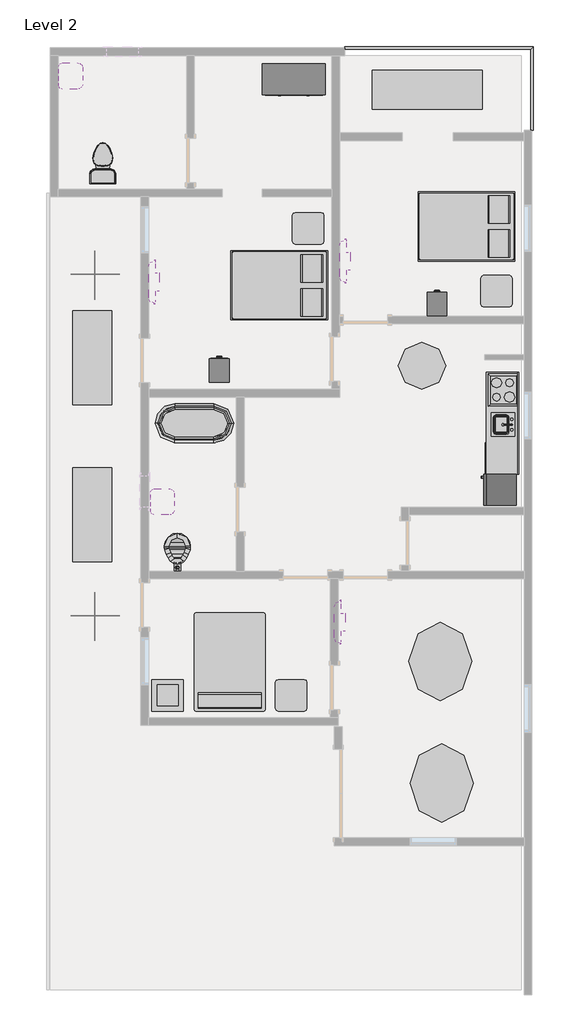
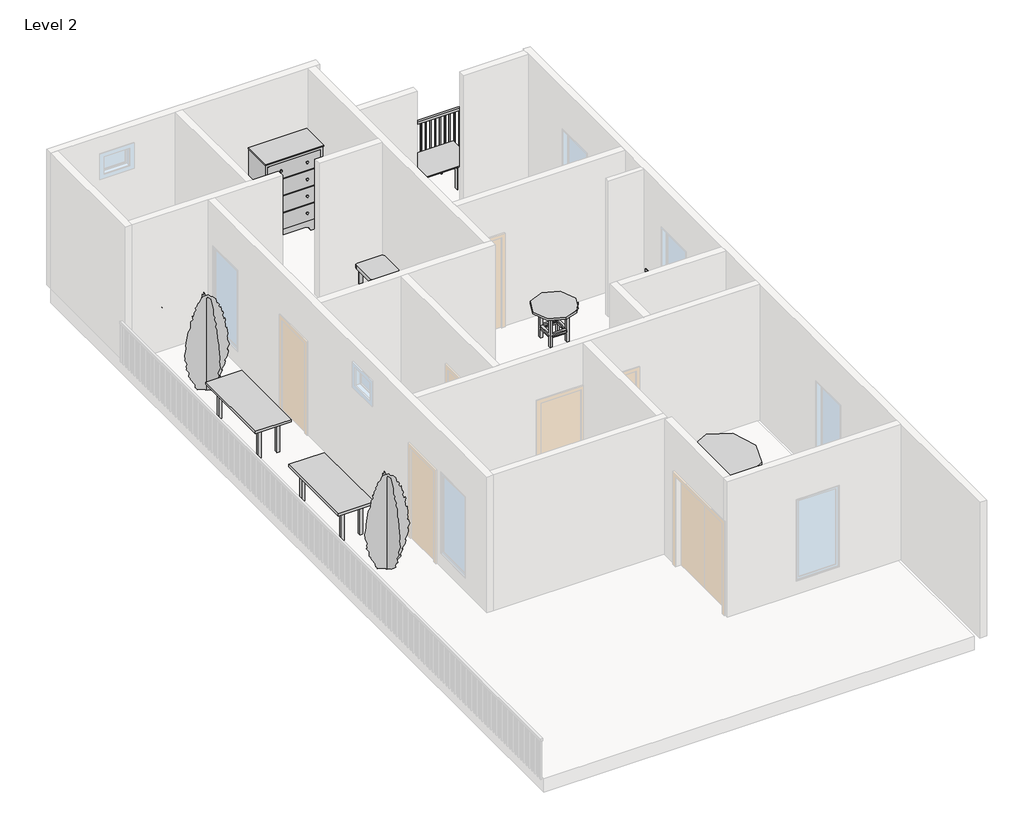
# One storey, part 4 of 4: 20 furniture elements, 6 flow terminals, 4 proxies, 2 geographic elements, 1 railing.
"""IFC4 building model written with IfcOpenShell, lengths in millimetres."""

from ifc_helpers import new_model, si_unit, frame, origin, place, context, project, spatial, polyline, outline, extrude, faceted_brep, transform, mapped, element, save
from components import proxy_a6faaae8, proxy_45b28599, kitchenette_medium_kitchenette_medium_844211aa, proxy_c523a7b7, flow_terminal_871c2e40, flow_terminal_62a433f7, flow_terminal_6d55091a, toilet_domestic_3d_toilet_domestic_3d_f7549cf7, toilet_domestic_3d_toilet_domestic_3d_183bbd19, flow_terminal_b374fae2, furniture_0810mm_56245f3a, furniture_c8abb964, furniture_0253826f, furniture_b1353b55, furniture_c6510c7c, furniture_9fa109b2, furniture_b5c51a22, furniture_92191dda, furniture_905aceb5, furniture_743965d2, furniture_bcf351fa, furniture_a5b052b6, rpc_tree_conifer_0001_chinese_juniper_7_1b9786cd

model = new_model("IFC4")

# Units and contexts
model_context = context("Model", 3, world=origin())
ifc_project = project(units=[si_unit("LENGTHUNIT", "METRE", prefix="MILLI")], contexts=[model_context])

# Site, building, storey
site = spatial("IfcSite", under=ifc_project)
building = spatial("IfcBuilding", under=site)
storey = spatial("IfcBuildingStorey", under=building, Name="Level 2", Elevation=3048.0)

# Proxies
placement = place(None, origin())
proxy_shape = proxy_a6faaae8(model_context)
element("IfcBuildingElementProxy", 1, Name="Cook Top-4 Unit2 : 22\" x 20\"", ObjectType="Cook Top-4 Unit2 : 22\" x 20\"", at=placement, inside=storey, context=model_context, shape_type="MappedRepresentation", body=[
    mapped(proxy_shape, transform((-3246.660887, 7038.0910469, 3048.0), x_axis=(0.0, -1.0, 0.0), y_axis=(1.0, 0.0, 0.0), z_axis=(0.0, 0.0, 1.0))),
])
proxy_2_shape = proxy_45b28599(model_context)
element("IfcBuildingElementProxy", 2, Name="Dishwasher : 24\" x 24\" x 34\"", ObjectType="Dishwasher : 24\" x 24\" x 34\"", at=placement, inside=storey, context=model_context, shape_type="MappedRepresentation", body=[
    mapped(proxy_2_shape, transform((-3538.5104518, 6086.9085154, 3048.0), x_axis=(0.0, -1.0, 0.0), y_axis=(1.0, 0.0, 0.0), z_axis=(0.0, 0.0, 1.0))),
])
kitchenette_medium_kitchenette_medium_shape = kitchenette_medium_kitchenette_medium_844211aa(model_context)
element("IfcBuildingElementProxy", 3, Name="Kitchenette - Medium : Kitchenette - Medium", ObjectType="Kitchenette - Medium : Kitchenette - Medium", at=placement, inside=storey, context=model_context, shape_type="MappedRepresentation", body=[
    mapped(kitchenette_medium_kitchenette_medium_shape, transform((-2941.860887, 6713.9287518, 3048.0), x_axis=(0.0, -1.0, 0.0), y_axis=(1.0, 0.0, 0.0), z_axis=(0.0, 0.0, 1.0))),
])
proxy_3_shape = proxy_c523a7b7(model_context)
element("IfcBuildingElementProxy", 4, Name="Refrigerator : 24\" x 25\" LH", ObjectType="Refrigerator : 24\" x 25\" LH", at=placement, inside=storey, context=model_context, shape_type="MappedRepresentation", body=[
    mapped(proxy_3_shape, transform((-3292.3098585, 5101.3410469, 3048.0), x_axis=(0.0, -1.0, 0.0), y_axis=(1.0, 0.0, 0.0), z_axis=(0.0, 0.0, 1.0))),
])

# Flow terminals
flow_terminal_shape = flow_terminal_871c2e40(model_context)
element("IfcFlowTerminal", 5, ObjectType="Sink Kitchen-Island : 18\" x 18\"", at=placement, inside=storey, context=model_context, shape_type="MappedRepresentation", body=[
    mapped(flow_terminal_shape, transform((-3249.0062881, 6380.6802875, 3033.6), x_axis=(0.0, -1.0, 0.0), y_axis=(1.0, 0.0, 0.0), z_axis=(0.0, 0.0, 1.0))),
])
flow_terminal_2_shape = flow_terminal_62a433f7(model_context)
element("IfcFlowTerminal", 6, ObjectType="Sink Vanity-Square : 20\" x 18\"", at=placement, inside=storey, context=model_context, shape_type="MappedRepresentation", body=[
    mapped(flow_terminal_2_shape, transform((-11689.8154859, 13118.4018063, 3962.4), x_axis=(0.0, 1.0000000000000002, 0.0), y_axis=(-1.0000000000000002, 0.0, 0.0), z_axis=(0.0, 0.0, 1.0))),
])
element("IfcFlowTerminal", 7, ObjectType="Sink Vanity-Square : 20\" x 18\"", at=placement, inside=storey, context=model_context, shape_type="MappedRepresentation", body=[
    mapped(flow_terminal_2_shape, transform((-9911.8154859, 4850.7018063, 3962.4), x_axis=(0.0, 1.0000000000000002, 0.0), y_axis=(-1.0000000000000002, 0.0, 0.0), z_axis=(0.0, 0.0, 1.0))),
])
flow_terminal_3_shape = flow_terminal_6d55091a(model_context)
element("IfcFlowTerminal", 8, ObjectType="Toilet-Commercial-Wall-3D : 15\" Seat Height", at=placement, inside=storey, context=model_context, shape_type="MappedRepresentation", body=[
    mapped(flow_terminal_3_shape, transform((-9976.1640408, 3443.9910469, 3048.0), x_axis=(1.0, 0.0, 0.0), y_axis=(0.0, 1.0, 0.0), z_axis=(0.0, 0.0, 1.0))),
])
toilet_domestic_3d_toilet_domestic_3d_shape = toilet_domestic_3d_toilet_domestic_3d_f7549cf7(model_context)
toilet_domestic_3d_toilet_domestic_3d_2_shape = toilet_domestic_3d_toilet_domestic_3d_183bbd19(model_context)
element("IfcFlowTerminal", 9, ObjectType="Toilet-Domestic-3D : Toilet-Domestic-3D", at=placement, inside=storey, context=model_context, shape_type="MappedRepresentation", body=[
    mapped(toilet_domestic_3d_toilet_domestic_3d_shape, transform((-11019.060887, 11533.2870743, 3048.0), x_axis=(-1.0000000000000004, 0.0, 0.0), y_axis=(0.0, -1.0000000000000004, 0.0), z_axis=(0.0, 0.0, 1.0))),
    mapped(toilet_domestic_3d_toilet_domestic_3d_2_shape, transform((-11019.060887, 11533.2870743, 3048.0), x_axis=(-1.0000000000000004, 0.0, 0.0), y_axis=(0.0, -1.0000000000000004, 0.0), z_axis=(0.0, 0.0, 1.0))),
])
flow_terminal_4_shape = flow_terminal_b374fae2(model_context)
element("IfcFlowTerminal", 10, ObjectType="Tub-Free Standing-3D : 30\" x 60\"", at=placement, inside=storey, context=model_context, shape_type="MappedRepresentation", body=[
    mapped(flow_terminal_4_shape, transform((-9241.060887, 6390.3910469, 3048.0), x_axis=(0.0, 1.0, 0.0), y_axis=(-1.0, 0.0, 0.0), z_axis=(0.0, 0.0, 1.0))),
])

# Furniture
furniture_0810mm_shape = furniture_0810mm_56245f3a(model_context)
element("IfcFurniture", 11, ObjectType="0810mm", at=placement, inside=storey, context=model_context, shape_type="MappedRepresentation", body=[
    mapped(furniture_0810mm_shape, transform((-6464.7222634, 2533.535561, 4267.2), x_axis=(0.0, 0.9999999999999998, 0.0), y_axis=(-0.9999999999999998, 0.0, 0.0), z_axis=(0.0, 0.0, 1.0))),
])
element("IfcFurniture", 12, ObjectType="0810mm", at=placement, inside=storey, context=model_context, shape_type="MappedRepresentation", body=[
    mapped(furniture_0810mm_shape, transform((-10071.5222634, 9137.535561, 4267.2), x_axis=(0.0, 0.9999999999999998, 0.0), y_axis=(-0.9999999999999998, 0.0, 0.0), z_axis=(0.0, 0.0, 1.0))),
])
element("IfcFurniture", 13, ObjectType="0810mm", at=placement, inside=storey, context=model_context, shape_type="MappedRepresentation", body=[
    mapped(furniture_0810mm_shape, transform((-6363.1222634, 9543.935561, 4267.2), x_axis=(0.0, 0.9999999999999998, 0.0), y_axis=(-0.9999999999999998, 0.0, 0.0), z_axis=(0.0, 0.0, 1.0))),
])
furniture_shape = furniture_c8abb964(model_context)
element("IfcFurniture", 14, ObjectType="Bed-Box : Double 53\" x 74\"", at=placement, inside=storey, context=model_context, shape_type="MappedRepresentation", body=[
    mapped(furniture_shape, transform((-7355.6313788, 9409.2435059, 3048.0), x_axis=(0.0, -1.0, 0.0), y_axis=(1.0, 0.0, 0.0), z_axis=(0.0, 0.0, 1.0))),
])
element("IfcFurniture", 15, ObjectType="Bed-Box : Double 53\" x 74\"", at=placement, inside=storey, context=model_context, shape_type="MappedRepresentation", body=[
    mapped(furniture_shape, transform((-3723.4313788, 10552.2435059, 3048.0), x_axis=(0.0, -1.0, 0.0), y_axis=(1.0, 0.0, 0.0), z_axis=(0.0, 0.0, 1.0))),
])
furniture_2_shape = furniture_0253826f(model_context)
element("IfcFurniture", 16, ObjectType="Bed-Standard : Double 54\" x 75\"", at=placement, inside=storey, context=model_context, shape_type="MappedRepresentation", body=[
    mapped(furniture_2_shape, transform((-8283.7723624, 1709.2959649, 3048.0), x_axis=(-1.0, 0.0, 0.0), y_axis=(0.0, -1.0, 0.0), z_axis=(0.0, 0.0, 1.0))),
])
furniture_3_shape = furniture_b1353b55(model_context)
element("IfcFurniture", 17, ObjectType="Cabinet-File 4 Drawer : 15\" x 18\"", at=placement, inside=storey, context=model_context, shape_type="MappedRepresentation", body=[
    mapped(furniture_3_shape, transform((-8886.3573341, 7276.9567468, 3048.0), x_axis=(-1.0000000000000007, 0.0, 0.0), y_axis=(0.0, -1.0000000000000007, 0.0), z_axis=(0.0, 0.0, 1.0))),
])
element("IfcFurniture", 18, ObjectType="Cabinet-File 4 Drawer : 15\" x 18\"", at=placement, inside=storey, context=model_context, shape_type="MappedRepresentation", body=[
    mapped(furniture_3_shape, transform((-4657.2573341, 8559.6567468, 3048.0), x_axis=(-1.0000000000000004, 0.0, 0.0), y_axis=(0.0, -1.0000000000000004, 0.0), z_axis=(0.0, 0.0, 1.0))),
])
furniture_4_shape = furniture_c6510c7c(model_context)
element("IfcFurniture", 19, ObjectType="Counter Top w Sink Hole : 24\" Depth", at=placement, inside=storey, context=model_context, shape_type="MappedRepresentation", body=[
    mapped(furniture_4_shape, transform((-2941.860887, 6180.5287518, 3033.6), x_axis=(0.0, -1.0, 0.0), y_axis=(1.0, 0.0, 0.0), z_axis=(0.0, 0.0, 1.0))),
])
furniture_5_shape = furniture_9fa109b2(model_context)
element("IfcFurniture", 20, ObjectType="Dresser : 48\" x 72\" x 24\"", at=placement, inside=storey, context=model_context, shape_type="MappedRepresentation", body=[
    mapped(furniture_5_shape, transform((-7041.4676272, 13433.754001, 3048.0), x_axis=(1.0, 0.0, 0.0), y_axis=(0.0, 1.0, 0.0), z_axis=(0.0, 0.0, 1.0))),
])
furniture_6_shape = furniture_b5c51a22(model_context)
element("IfcFurniture", 21, ObjectType="Table-Coffee : 24\" x 24\" x 24\"", at=placement, inside=storey, context=model_context, shape_type="MappedRepresentation", body=[
    mapped(furniture_6_shape, transform((-9780.0266537, 1011.9799691, 3048.0), x_axis=(1.0, 0.0, 0.0), y_axis=(0.0, 1.0, 0.0), z_axis=(0.0, 0.0, 1.0))),
])
furniture_7_shape = furniture_92191dda(model_context)
element("IfcFurniture", 22, ObjectType="Table-Dining : 30\" x 84\" x 22\"", at=placement, inside=storey, context=model_context, shape_type="MappedRepresentation", body=[
    mapped(furniture_7_shape, transform((-4738.1266537, 12772.1799691, 3048.0), x_axis=(1.0, 0.0, 0.0), y_axis=(0.0, 1.0, 0.0), z_axis=(0.0, 0.0, 1.0))),
])
furniture_8_shape = furniture_905aceb5(model_context)
element("IfcFurniture", 23, ObjectType="Table-Dining Round w Chairs : 36\" Diameter", at=placement, inside=storey, context=model_context, shape_type="MappedRepresentation", body=[
    mapped(furniture_8_shape, transform((-4925.1428542, 7692.8697354, 3048.0), x_axis=(1.0, 0.0, 0.0), y_axis=(0.0, 1.0, 0.0), z_axis=(0.0, 0.0, 1.0))),
])
furniture_9_shape = furniture_743965d2(model_context)
element("IfcFurniture", 24, ObjectType="Table-Ellipse : 60\" x 48\"", at=placement, inside=storey, context=model_context, shape_type="MappedRepresentation", body=[
    mapped(furniture_9_shape, transform((-4465.860887, 1767.5910469, 3048.0), x_axis=(0.0, 1.0000000000000002, 0.0), y_axis=(-1.0000000000000002, 0.0, 0.0), z_axis=(0.0, 0.0, 1.0))),
])
element("IfcFurniture", 25, ObjectType="Table-Ellipse : 60\" x 48\"", at=placement, inside=storey, context=model_context, shape_type="MappedRepresentation", body=[
    mapped(furniture_9_shape, transform((-4440.460887, -594.6089531, 3048.0), x_axis=(0.0, 1.0000000000000002, 0.0), y_axis=(-1.0000000000000002, 0.0, 0.0), z_axis=(0.0, 0.0, 1.0))),
])
furniture_10_shape = furniture_bcf351fa(model_context)
element("IfcFurniture", 26, ObjectType="Table-End : 24\" x 24\"", at=placement, inside=storey, context=model_context, shape_type="MappedRepresentation", body=[
    mapped(furniture_10_shape, transform((-3682.1945173, 8803.3910469, 3048.0), x_axis=(1.0, 0.0, 0.0), y_axis=(0.0, 1.0, 0.0), z_axis=(0.0, 0.0, 1.0))),
])
element("IfcFurniture", 27, ObjectType="Table-End : 24\" x 24\"", at=placement, inside=storey, context=model_context, shape_type="MappedRepresentation", body=[
    mapped(furniture_10_shape, transform((-7339.7945173, 10022.5910469, 3048.0), x_axis=(1.0, 0.0, 0.0), y_axis=(0.0, 1.0, 0.0), z_axis=(0.0, 0.0, 1.0))),
])
element("IfcFurniture", 28, ObjectType="Table-End : 24\" x 24\"", at=placement, inside=storey, context=model_context, shape_type="MappedRepresentation", body=[
    mapped(furniture_10_shape, transform((-7669.9945173, 954.7910469, 3048.0), x_axis=(1.0, 0.0, 0.0), y_axis=(0.0, 1.0, 0.0), z_axis=(0.0, 0.0, 1.0))),
])
furniture_11_shape = furniture_a5b052b6(model_context)
element("IfcFurniture", 29, ObjectType="Table-Rectangular : 72\" x 30\"", at=placement, inside=storey, context=model_context, shape_type="MappedRepresentation", body=[
    mapped(furniture_11_shape, transform((-11222.260887, 7660.3910469, 3048.0), x_axis=(0.0, 1.0, 0.0), y_axis=(-1.0, 0.0, 0.0), z_axis=(0.0, 0.0, 1.0))),
])
element("IfcFurniture", 30, ObjectType="Table-Rectangular : 72\" x 30\"", at=placement, inside=storey, context=model_context, shape_type="MappedRepresentation", body=[
    mapped(furniture_11_shape, transform((-11222.260887, 4612.3910469, 3048.0), x_axis=(0.0, 1.0000000000000002, 0.0), y_axis=(-1.0000000000000002, 0.0, 0.0), z_axis=(0.0, 0.0, 1.0))),
])

# Geographic elements
rpc_tree_conifer_0001_chinese_juniper_7_shape = rpc_tree_conifer_0001_chinese_juniper_7_1b9786cd(model_context)
element("IfcGeographicElement", 31, ObjectType="RPC Tree - Conifer.0001 : Chinese Juniper - 7'", at=placement, inside=storey, context=model_context, shape_type="MappedRepresentation", body=[
    mapped(rpc_tree_conifer_0001_chinese_juniper_7_shape, transform((-11171.6575581, 9285.9910469, 3048.0), x_axis=(1.0, 0.0, 0.0), y_axis=(0.0, 1.0, 0.0), z_axis=(0.0, 0.0, 1.0))),
])
element("IfcGeographicElement", 32, ObjectType="RPC Tree - Conifer.0001 : Chinese Juniper - 7'", at=placement, inside=storey, context=model_context, shape_type="MappedRepresentation", body=[
    mapped(rpc_tree_conifer_0001_chinese_juniper_7_shape, transform((-11171.6575581, 2656.5910469, 3048.0), x_axis=(1.0, 0.0, 0.0), y_axis=(0.0, 1.0, 0.0), z_axis=(0.0, 0.0, 1.0))),
])

# Railing
element("IfcRailing", 33, ObjectType="Handrail - Rectangular", at=placement, inside=storey, context=model_context, shape_type="SolidModel", body=[
    faceted_brep([(-6320.060887, 13705.5910469, 3962.4), (-6320.060887, 13705.5910469, 3911.6), (-6320.060887, 13654.7910469, 3911.6), (-6320.060887, 13654.7910469, 3962.4), (-2662.460887, 13705.5910469, 3962.4), (-2662.460887, 13705.5910469, 3911.6), (-2713.260887, 13654.7910469, 3911.6), (-2713.260887, 13654.7910469, 3962.4), (-2662.460887, 12079.9910469, 3962.4), (-2713.260887, 12079.9910469, 3962.4), (-2713.260887, 12079.9910469, 3911.6), (-2662.460887, 12079.9910469, 3911.6)], [[[0, 1, 2, 3]], [[1, 0, 4, 5]], [[2, 1, 5, 6]], [[3, 2, 6, 7]], [[0, 3, 7, 4]], [[8, 9, 10, 11]], [[5, 4, 8, 11]], [[6, 5, 11, 10]], [[7, 6, 10, 9]], [[4, 7, 9, 8]]]),
    extrude(outline(polyline([(-2697.385887, 12165.7160469), (-2678.335887, 12165.7160469), (-2678.335887, 12146.6660469), (-2697.385887, 12146.6660469), (-2697.385887, 12165.7160469)])), frame((0.0, 0.0, 3048.0), z_axis=(0.0, 0.0, 1.0), x_axis=(1.0, 0.0, 0.0)), (0.0, 0.0, 1.0), 863.6),
    extrude(outline(polyline([(-2697.385887, 12267.3160469), (-2678.335887, 12267.3160469), (-2678.335887, 12248.2660469), (-2697.385887, 12248.2660469), (-2697.385887, 12267.3160469)])), frame((0.0, 0.0, 3048.0), z_axis=(0.0, 0.0, 1.0), x_axis=(1.0, 0.0, 0.0)), (0.0, 0.0, 1.0), 863.6),
    extrude(outline(polyline([(-2697.385887, 12368.9160469), (-2678.335887, 12368.9160469), (-2678.335887, 12349.8660469), (-2697.385887, 12349.8660469), (-2697.385887, 12368.9160469)])), frame((0.0, 0.0, 3048.0), z_axis=(0.0, 0.0, 1.0), x_axis=(1.0, 0.0, 0.0)), (0.0, 0.0, 1.0), 863.6),
    extrude(outline(polyline([(-2697.385887, 12470.5160469), (-2678.335887, 12470.5160469), (-2678.335887, 12451.4660469), (-2697.385887, 12451.4660469), (-2697.385887, 12470.5160469)])), frame((0.0, 0.0, 3048.0), z_axis=(0.0, 0.0, 1.0), x_axis=(1.0, 0.0, 0.0)), (0.0, 0.0, 1.0), 863.6),
    extrude(outline(polyline([(-2697.385887, 12572.1160469), (-2678.335887, 12572.1160469), (-2678.335887, 12553.0660469), (-2697.385887, 12553.0660469), (-2697.385887, 12572.1160469)])), frame((0.0, 0.0, 3048.0), z_axis=(0.0, 0.0, 1.0), x_axis=(1.0, 0.0, 0.0)), (0.0, 0.0, 1.0), 863.6),
    extrude(outline(polyline([(-2697.385887, 12673.7160469), (-2678.335887, 12673.7160469), (-2678.335887, 12654.6660469), (-2697.385887, 12654.6660469), (-2697.385887, 12673.7160469)])), frame((0.0, 0.0, 3048.0), z_axis=(0.0, 0.0, 1.0), x_axis=(1.0, 0.0, 0.0)), (0.0, 0.0, 1.0), 863.6),
    extrude(outline(polyline([(-2697.385887, 12775.3160469), (-2678.335887, 12775.3160469), (-2678.335887, 12756.2660469), (-2697.385887, 12756.2660469), (-2697.385887, 12775.3160469)])), frame((0.0, 0.0, 3048.0), z_axis=(0.0, 0.0, 1.0), x_axis=(1.0, 0.0, 0.0)), (0.0, 0.0, 1.0), 863.6),
    extrude(outline(polyline([(-2697.385887, 12876.9160469), (-2678.335887, 12876.9160469), (-2678.335887, 12857.8660469), (-2697.385887, 12857.8660469), (-2697.385887, 12876.9160469)])), frame((0.0, 0.0, 3048.0), z_axis=(0.0, 0.0, 1.0), x_axis=(1.0, 0.0, 0.0)), (0.0, 0.0, 1.0), 863.6),
    extrude(outline(polyline([(-2697.385887, 12978.5160469), (-2678.335887, 12978.5160469), (-2678.335887, 12959.4660469), (-2697.385887, 12959.4660469), (-2697.385887, 12978.5160469)])), frame((0.0, 0.0, 3048.0), z_axis=(0.0, 0.0, 1.0), x_axis=(1.0, 0.0, 0.0)), (0.0, 0.0, 1.0), 863.6),
    extrude(outline(polyline([(-2697.385887, 13080.1160469), (-2678.335887, 13080.1160469), (-2678.335887, 13061.0660469), (-2697.385887, 13061.0660469), (-2697.385887, 13080.1160469)])), frame((0.0, 0.0, 3048.0), z_axis=(0.0, 0.0, 1.0), x_axis=(1.0, 0.0, 0.0)), (0.0, 0.0, 1.0), 863.6),
    extrude(outline(polyline([(-2697.385887, 13181.7160469), (-2678.335887, 13181.7160469), (-2678.335887, 13162.6660469), (-2697.385887, 13162.6660469), (-2697.385887, 13181.7160469)])), frame((0.0, 0.0, 3048.0), z_axis=(0.0, 0.0, 1.0), x_axis=(1.0, 0.0, 0.0)), (0.0, 0.0, 1.0), 863.6),
    extrude(outline(polyline([(-2697.385887, 13283.3160469), (-2678.335887, 13283.3160469), (-2678.335887, 13264.2660469), (-2697.385887, 13264.2660469), (-2697.385887, 13283.3160469)])), frame((0.0, 0.0, 3048.0), z_axis=(0.0, 0.0, 1.0), x_axis=(1.0, 0.0, 0.0)), (0.0, 0.0, 1.0), 863.6),
    extrude(outline(polyline([(-2697.385887, 13384.9160469), (-2678.335887, 13384.9160469), (-2678.335887, 13365.8660469), (-2697.385887, 13365.8660469), (-2697.385887, 13384.9160469)])), frame((0.0, 0.0, 3048.0), z_axis=(0.0, 0.0, 1.0), x_axis=(1.0, 0.0, 0.0)), (0.0, 0.0, 1.0), 863.6),
    extrude(outline(polyline([(-2697.385887, 13486.5160469), (-2678.335887, 13486.5160469), (-2678.335887, 13467.4660469), (-2697.385887, 13467.4660469), (-2697.385887, 13486.5160469)])), frame((0.0, 0.0, 3048.0), z_axis=(0.0, 0.0, 1.0), x_axis=(1.0, 0.0, 0.0)), (0.0, 0.0, 1.0), 863.6),
    extrude(outline(polyline([(-2697.385887, 13588.1160469), (-2678.335887, 13588.1160469), (-2678.335887, 13569.0660469), (-2697.385887, 13569.0660469), (-2697.385887, 13588.1160469)])), frame((0.0, 0.0, 3048.0), z_axis=(0.0, 0.0, 1.0), x_axis=(1.0, 0.0, 0.0)), (0.0, 0.0, 1.0), 863.6),
    extrude(outline(polyline([(-2773.585887, 13670.6660469), (-2773.585887, 13689.7160469), (-2754.535887, 13689.7160469), (-2754.535887, 13670.6660469), (-2773.585887, 13670.6660469)])), frame((0.0, 0.0, 3048.0), z_axis=(0.0, 0.0, 1.0), x_axis=(1.0, 0.0, 0.0)), (0.0, 0.0, 1.0), 863.6),
    extrude(outline(polyline([(-2875.185887, 13670.6660469), (-2875.185887, 13689.7160469), (-2856.135887, 13689.7160469), (-2856.135887, 13670.6660469), (-2875.185887, 13670.6660469)])), frame((0.0, 0.0, 3048.0), z_axis=(0.0, 0.0, 1.0), x_axis=(1.0, 0.0, 0.0)), (0.0, 0.0, 1.0), 863.6),
    extrude(outline(polyline([(-2976.785887, 13670.6660469), (-2976.785887, 13689.7160469), (-2957.735887, 13689.7160469), (-2957.735887, 13670.6660469), (-2976.785887, 13670.6660469)])), frame((0.0, 0.0, 3048.0), z_axis=(0.0, 0.0, 1.0), x_axis=(1.0, 0.0, 0.0)), (0.0, 0.0, 1.0), 863.6),
    extrude(outline(polyline([(-3078.385887, 13670.6660469), (-3078.385887, 13689.7160469), (-3059.335887, 13689.7160469), (-3059.335887, 13670.6660469), (-3078.385887, 13670.6660469)])), frame((0.0, 0.0, 3048.0), z_axis=(0.0, 0.0, 1.0), x_axis=(1.0, 0.0, 0.0)), (0.0, 0.0, 1.0), 863.6),
    extrude(outline(polyline([(-3179.985887, 13670.6660469), (-3179.985887, 13689.7160469), (-3160.935887, 13689.7160469), (-3160.935887, 13670.6660469), (-3179.985887, 13670.6660469)])), frame((0.0, 0.0, 3048.0), z_axis=(0.0, 0.0, 1.0), x_axis=(1.0, 0.0, 0.0)), (0.0, 0.0, 1.0), 863.6),
    extrude(outline(polyline([(-3281.585887, 13670.6660469), (-3281.585887, 13689.7160469), (-3262.535887, 13689.7160469), (-3262.535887, 13670.6660469), (-3281.585887, 13670.6660469)])), frame((0.0, 0.0, 3048.0), z_axis=(0.0, 0.0, 1.0), x_axis=(1.0, 0.0, 0.0)), (0.0, 0.0, 1.0), 863.6),
    extrude(outline(polyline([(-3383.185887, 13670.6660469), (-3383.185887, 13689.7160469), (-3364.135887, 13689.7160469), (-3364.135887, 13670.6660469), (-3383.185887, 13670.6660469)])), frame((0.0, 0.0, 3048.0), z_axis=(0.0, 0.0, 1.0), x_axis=(1.0, 0.0, 0.0)), (0.0, 0.0, 1.0), 863.6),
    extrude(outline(polyline([(-3484.785887, 13670.6660469), (-3484.785887, 13689.7160469), (-3465.735887, 13689.7160469), (-3465.735887, 13670.6660469), (-3484.785887, 13670.6660469)])), frame((0.0, 0.0, 3048.0), z_axis=(0.0, 0.0, 1.0), x_axis=(1.0, 0.0, 0.0)), (0.0, 0.0, 1.0), 863.6),
    extrude(outline(polyline([(-3586.385887, 13670.6660469), (-3586.385887, 13689.7160469), (-3567.335887, 13689.7160469), (-3567.335887, 13670.6660469), (-3586.385887, 13670.6660469)])), frame((0.0, 0.0, 3048.0), z_axis=(0.0, 0.0, 1.0), x_axis=(1.0, 0.0, 0.0)), (0.0, 0.0, 1.0), 863.6),
    extrude(outline(polyline([(-3687.985887, 13670.6660469), (-3687.985887, 13689.7160469), (-3668.935887, 13689.7160469), (-3668.935887, 13670.6660469), (-3687.985887, 13670.6660469)])), frame((0.0, 0.0, 3048.0), z_axis=(0.0, 0.0, 1.0), x_axis=(1.0, 0.0, 0.0)), (0.0, 0.0, 1.0), 863.6),
    extrude(outline(polyline([(-3789.585887, 13670.6660469), (-3789.585887, 13689.7160469), (-3770.535887, 13689.7160469), (-3770.535887, 13670.6660469), (-3789.585887, 13670.6660469)])), frame((0.0, 0.0, 3048.0), z_axis=(0.0, 0.0, 1.0), x_axis=(1.0, 0.0, 0.0)), (0.0, 0.0, 1.0), 863.6),
    extrude(outline(polyline([(-3891.185887, 13670.6660469), (-3891.185887, 13689.7160469), (-3872.135887, 13689.7160469), (-3872.135887, 13670.6660469), (-3891.185887, 13670.6660469)])), frame((0.0, 0.0, 3048.0), z_axis=(0.0, 0.0, 1.0), x_axis=(1.0, 0.0, 0.0)), (0.0, 0.0, 1.0), 863.6),
    extrude(outline(polyline([(-3992.785887, 13670.6660469), (-3992.785887, 13689.7160469), (-3973.735887, 13689.7160469), (-3973.735887, 13670.6660469), (-3992.785887, 13670.6660469)])), frame((0.0, 0.0, 3048.0), z_axis=(0.0, 0.0, 1.0), x_axis=(1.0, 0.0, 0.0)), (0.0, 0.0, 1.0), 863.6),
    extrude(outline(polyline([(-4094.385887, 13670.6660469), (-4094.385887, 13689.7160469), (-4075.335887, 13689.7160469), (-4075.335887, 13670.6660469), (-4094.385887, 13670.6660469)])), frame((0.0, 0.0, 3048.0), z_axis=(0.0, 0.0, 1.0), x_axis=(1.0, 0.0, 0.0)), (0.0, 0.0, 1.0), 863.6),
    extrude(outline(polyline([(-4195.985887, 13670.6660469), (-4195.985887, 13689.7160469), (-4176.935887, 13689.7160469), (-4176.935887, 13670.6660469), (-4195.985887, 13670.6660469)])), frame((0.0, 0.0, 3048.0), z_axis=(0.0, 0.0, 1.0), x_axis=(1.0, 0.0, 0.0)), (0.0, 0.0, 1.0), 863.6),
    extrude(outline(polyline([(-4297.585887, 13670.6660469), (-4297.585887, 13689.7160469), (-4278.535887, 13689.7160469), (-4278.535887, 13670.6660469), (-4297.585887, 13670.6660469)])), frame((0.0, 0.0, 3048.0), z_axis=(0.0, 0.0, 1.0), x_axis=(1.0, 0.0, 0.0)), (0.0, 0.0, 1.0), 863.6),
    extrude(outline(polyline([(-4399.185887, 13670.6660469), (-4399.185887, 13689.7160469), (-4380.135887, 13689.7160469), (-4380.135887, 13670.6660469), (-4399.185887, 13670.6660469)])), frame((0.0, 0.0, 3048.0), z_axis=(0.0, 0.0, 1.0), x_axis=(1.0, 0.0, 0.0)), (0.0, 0.0, 1.0), 863.6),
    extrude(outline(polyline([(-4500.785887, 13670.6660469), (-4500.785887, 13689.7160469), (-4481.735887, 13689.7160469), (-4481.735887, 13670.6660469), (-4500.785887, 13670.6660469)])), frame((0.0, 0.0, 3048.0), z_axis=(0.0, 0.0, 1.0), x_axis=(1.0, 0.0, 0.0)), (0.0, 0.0, 1.0), 863.6),
    extrude(outline(polyline([(-4602.385887, 13670.6660469), (-4602.385887, 13689.7160469), (-4583.335887, 13689.7160469), (-4583.335887, 13670.6660469), (-4602.385887, 13670.6660469)])), frame((0.0, 0.0, 3048.0), z_axis=(0.0, 0.0, 1.0), x_axis=(1.0, 0.0, 0.0)), (0.0, 0.0, 1.0), 863.6),
    extrude(outline(polyline([(-4703.985887, 13670.6660469), (-4703.985887, 13689.7160469), (-4684.935887, 13689.7160469), (-4684.935887, 13670.6660469), (-4703.985887, 13670.6660469)])), frame((0.0, 0.0, 3048.0), z_axis=(0.0, 0.0, 1.0), x_axis=(1.0, 0.0, 0.0)), (0.0, 0.0, 1.0), 863.6),
    extrude(outline(polyline([(-4805.585887, 13670.6660469), (-4805.585887, 13689.7160469), (-4786.535887, 13689.7160469), (-4786.535887, 13670.6660469), (-4805.585887, 13670.6660469)])), frame((0.0, 0.0, 3048.0), z_axis=(0.0, 0.0, 1.0), x_axis=(1.0, 0.0, 0.0)), (0.0, 0.0, 1.0), 863.6),
    extrude(outline(polyline([(-4907.185887, 13670.6660469), (-4907.185887, 13689.7160469), (-4888.135887, 13689.7160469), (-4888.135887, 13670.6660469), (-4907.185887, 13670.6660469)])), frame((0.0, 0.0, 3048.0), z_axis=(0.0, 0.0, 1.0), x_axis=(1.0, 0.0, 0.0)), (0.0, 0.0, 1.0), 863.6),
    extrude(outline(polyline([(-5008.785887, 13670.6660469), (-5008.785887, 13689.7160469), (-4989.735887, 13689.7160469), (-4989.735887, 13670.6660469), (-5008.785887, 13670.6660469)])), frame((0.0, 0.0, 3048.0), z_axis=(0.0, 0.0, 1.0), x_axis=(1.0, 0.0, 0.0)), (0.0, 0.0, 1.0), 863.6),
    extrude(outline(polyline([(-5110.385887, 13670.6660469), (-5110.385887, 13689.7160469), (-5091.335887, 13689.7160469), (-5091.335887, 13670.6660469), (-5110.385887, 13670.6660469)])), frame((0.0, 0.0, 3048.0), z_axis=(0.0, 0.0, 1.0), x_axis=(1.0, 0.0, 0.0)), (0.0, 0.0, 1.0), 863.6),
    extrude(outline(polyline([(-5211.985887, 13670.6660469), (-5211.985887, 13689.7160469), (-5192.935887, 13689.7160469), (-5192.935887, 13670.6660469), (-5211.985887, 13670.6660469)])), frame((0.0, 0.0, 3048.0), z_axis=(0.0, 0.0, 1.0), x_axis=(1.0, 0.0, 0.0)), (0.0, 0.0, 1.0), 863.6),
    extrude(outline(polyline([(-5313.585887, 13670.6660469), (-5313.585887, 13689.7160469), (-5294.535887, 13689.7160469), (-5294.535887, 13670.6660469), (-5313.585887, 13670.6660469)])), frame((0.0, 0.0, 3048.0), z_axis=(0.0, 0.0, 1.0), x_axis=(1.0, 0.0, 0.0)), (0.0, 0.0, 1.0), 863.6),
    extrude(outline(polyline([(-5415.185887, 13670.6660469), (-5415.185887, 13689.7160469), (-5396.135887, 13689.7160469), (-5396.135887, 13670.6660469), (-5415.185887, 13670.6660469)])), frame((0.0, 0.0, 3048.0), z_axis=(0.0, 0.0, 1.0), x_axis=(1.0, 0.0, 0.0)), (0.0, 0.0, 1.0), 863.6),
    extrude(outline(polyline([(-5516.785887, 13670.6660469), (-5516.785887, 13689.7160469), (-5497.735887, 13689.7160469), (-5497.735887, 13670.6660469), (-5516.785887, 13670.6660469)])), frame((0.0, 0.0, 3048.0), z_axis=(0.0, 0.0, 1.0), x_axis=(1.0, 0.0, 0.0)), (0.0, 0.0, 1.0), 863.6),
    extrude(outline(polyline([(-5618.385887, 13670.6660469), (-5618.385887, 13689.7160469), (-5599.335887, 13689.7160469), (-5599.335887, 13670.6660469), (-5618.385887, 13670.6660469)])), frame((0.0, 0.0, 3048.0), z_axis=(0.0, 0.0, 1.0), x_axis=(1.0, 0.0, 0.0)), (0.0, 0.0, 1.0), 863.6),
    extrude(outline(polyline([(-5719.985887, 13670.6660469), (-5719.985887, 13689.7160469), (-5700.935887, 13689.7160469), (-5700.935887, 13670.6660469), (-5719.985887, 13670.6660469)])), frame((0.0, 0.0, 3048.0), z_axis=(0.0, 0.0, 1.0), x_axis=(1.0, 0.0, 0.0)), (0.0, 0.0, 1.0), 863.6),
    extrude(outline(polyline([(-5821.585887, 13670.6660469), (-5821.585887, 13689.7160469), (-5802.535887, 13689.7160469), (-5802.535887, 13670.6660469), (-5821.585887, 13670.6660469)])), frame((0.0, 0.0, 3048.0), z_axis=(0.0, 0.0, 1.0), x_axis=(1.0, 0.0, 0.0)), (0.0, 0.0, 1.0), 863.6),
    extrude(outline(polyline([(-5923.185887, 13670.6660469), (-5923.185887, 13689.7160469), (-5904.135887, 13689.7160469), (-5904.135887, 13670.6660469), (-5923.185887, 13670.6660469)])), frame((0.0, 0.0, 3048.0), z_axis=(0.0, 0.0, 1.0), x_axis=(1.0, 0.0, 0.0)), (0.0, 0.0, 1.0), 863.6),
    extrude(outline(polyline([(-6024.785887, 13670.6660469), (-6024.785887, 13689.7160469), (-6005.735887, 13689.7160469), (-6005.735887, 13670.6660469), (-6024.785887, 13670.6660469)])), frame((0.0, 0.0, 3048.0), z_axis=(0.0, 0.0, 1.0), x_axis=(1.0, 0.0, 0.0)), (0.0, 0.0, 1.0), 863.6),
    extrude(outline(polyline([(-6126.385887, 13670.6660469), (-6126.385887, 13689.7160469), (-6107.335887, 13689.7160469), (-6107.335887, 13670.6660469), (-6126.385887, 13670.6660469)])), frame((0.0, 0.0, 3048.0), z_axis=(0.0, 0.0, 1.0), x_axis=(1.0, 0.0, 0.0)), (0.0, 0.0, 1.0), 863.6),
    extrude(outline(polyline([(-6227.985887, 13670.6660469), (-6227.985887, 13689.7160469), (-6208.935887, 13689.7160469), (-6208.935887, 13670.6660469), (-6227.985887, 13670.6660469)])), frame((0.0, 0.0, 3048.0), z_axis=(0.0, 0.0, 1.0), x_axis=(1.0, 0.0, 0.0)), (0.0, 0.0, 1.0), 863.6),
    extrude(outline(polyline([(-2697.385887, 13670.6660469), (-2697.385887, 13689.7160469), (-2678.335887, 13689.7160469), (-2678.335887, 13670.6660469), (-2697.385887, 13670.6660469)])), frame((0.0, 0.0, 3048.0), z_axis=(0.0, 0.0, 1.0), x_axis=(1.0, 0.0, 0.0)), (0.0, 0.0, 1.0), 863.6),
    extrude(outline(polyline([(-2697.385887, 12099.0410469), (-2678.335887, 12099.0410469), (-2678.335887, 12079.9910469), (-2697.385887, 12079.9910469), (-2697.385887, 12099.0410469)])), frame((0.0, 0.0, 3048.0), z_axis=(0.0, 0.0, 1.0), x_axis=(1.0, 0.0, 0.0)), (0.0, 0.0, 1.0), 863.6),
    extrude(outline(polyline([(-6320.060887, 13670.6660469), (-6320.060887, 13689.7160469), (-6301.010887, 13689.7160469), (-6301.010887, 13670.6660469), (-6320.060887, 13670.6660469)])), frame((0.0, 0.0, 3048.0), z_axis=(0.0, 0.0, 1.0), x_axis=(1.0, 0.0, 0.0)), (0.0, 0.0, 1.0), 863.6),
])

save(model, "model.ifc")

# Revit data of these elements
# Type "Cook Top-4 Unit2 : 22\" x 20\""
#   Depth = 1' - 8"
#   Width = 1' - 10"
#   Burner Material = Steel, Chrome Plated
#   Cooktop Material = Steel, Polished
#   Default Elevation = 0
#   Assembly Code = ""
# Type "Dishwasher : 24\" x 24\" x 34\""
#   Label = "DW"
#   Assembly Code = "E1090400"
#   Depth = 2' - 0"
#   Height = 2' - 10"
#   Width = 2' - 0"
#   Dishwasher Material = Steel, Paint Finish, Ivory, Glossy
#   Panel Face Material = Plastic, Opaque Black
#   Default Elevation = 0
# Type "Kitchenette - Medium : Kitchenette - Medium"
#   Assembly Code = "E1090400"
#   Counter Length = 6' - 6"
#   Cabinet Width = 4' - 6"
#   Cabinet Height = 2' - 10 1/2"
#   Cabinet Depth = 2' - 0"
#   Toe Depth = 0' - 3"
#   Toe Height = 0' - 3 1/2"
#   Cabinet Material = Cabinets
#   Door/Drawer Material = Cabinets
#   Handle Material = Cabinets - Handles
#   Default Elevation = 0
# Type "Refrigerator : 24\" x 25\" LH"
#   Label = "REF."
#   Assembly Code = "E1090400"
#   Depth = 2' - 0 3/4"
#   Handle = 0' - 1 1/2"
#   Height = 5' - 3 1/2"
#   Rear Clearance = 0' - 2"
#   Top Door Height = 1' - 8"
#   Width = 1' - 11 1/2"
#   Material = Steel, Paint Finish, Ivory, Glossy
#   Default Elevation = 0
# Type "Sink Kitchen-Island : 18\" x 18\""
#   Assembly Code = "D2010410"
#   Counter Height = 3' - 0"
#   Depth = 1' - 6"
#   Width = 1' - 6"
#   Faucet Material = Steel, Polished
#   Sink Material = Steel, Polished
#   Default Elevation = 0
# Type "Sink Vanity-Square : 20\" x 18\""
#   Assembly Code = "D2010400"
#   Counter Height = 2' - 7"
#   Depth = 1' - 6"
#   Width = 1' - 8"
#   Basin Material = Porcelain, Linen
#   Faucet Material = Steel, Polished
#   Default Elevation = 0
# Type "Toilet-Commercial-Wall-3D : 15\" Seat Height"
#   Assembly Code = "D2010110"
#   Mounting Height = 1' - 3"
#   Piping Material = Steel, Polished
#   Toilet - Bowl Material = Porcelain, Ivory
#   Toilet - Seat Material = Laminate, Ivory, Matte
#   Default Elevation = 0
# Type "Toilet-Domestic-3D : Toilet-Domestic-3D"
#   Assembly Code = "D2010110"
#   Toilet - Bowl/Basin Material = Porcelain, Linen
#   Toilet - Seat Material = Laminate, Linen, Matte
#   Default Elevation = 0
# Type "Tub-Free Standing-3D : 30\" x 60\""
#   Assembly Code = "D2010110"
#   Height = 1' - 6"
#   Length = 5' - 0"
#   Width = 2' - 6"
#   Tub Material = Porcelain, Ivory
#   Default Elevation = 0
# Type "0810mm"
#   SinAng = 0' - 0.0193"
#   L = 2' - 3.79372"
#   H = 1' - 3.6354"
#   Thickness = 0' - 4.33071"
#   Diagonal = 2' - 7.88976"
#   CosAng = 0' - 0.03431"
#   Stand [instance default] = yes
#   Default Elevation = 0
# Type "Bed-Box : Double 53\" x 74\""
#   Assembly Code = "E2020200"
#   Length = 6' - 2"
#   Width = 4' - 5"
#   Frame Material = Birch
#   Mattress Material = Linen, White
#   Default Elevation = 0
# Type "Bed-Standard : Double 54\" x 75\""
#   Assembly Code = "E2020200"
#   Length = 6' - 3"
#   Width = 4' - 6"
#   Leg Material = Steel, Chrome Plated
#   Mattress Material = Linen, White
#   Default Elevation = 0
# Type "Cabinet-File 4 Drawer : 15\" x 18\""
#   Assembly Code = "E2020200"
#   Depth = 1' - 6"
#   Height = 4' - 4"
#   Width = 1' - 3"
#   Cabinet Material = Steel, Paint Finish, Ivory, Glossy
#   Handle Material = Steel, Chrome Plated
#   Default Elevation = 0
# Type "Counter Top w Sink Hole : 24\" Depth"
#   Assembly Code = "C1030400"
#   Counter Thickness = 0' - 1 1/2"
#   Depth = 2' - 1"
#   Height = 3' - 0"
#   Length [instance default] = 8' - 0"
#   Sink Location [instance default] = 2' - 0"
#   Sink Location To Wall [instance default] = 0' - 6"
#   Sink Opening Depth [instance default] = 1' - 3"
#   Sink Opening Width [instance default] = 2' - 3"
#   Counter Top Material = none
#   Default Elevation = 0
# Type "Dresser : 48\" x 72\" x 24\""
#   Assembly Code = "E2020200"
#   Depth = 2' - 0"
#   Height = 6' - 0"
#   Width = 4' - 0"
#   Dresser Material = Laminate - Ivory, Glossy
#   Drawer Material = Laminate, Ivory, Matte
#   Knob Material = Cherry
#   Default Elevation = 0
# Type "Table-Coffee : 24\" x 24\" x 24\""
#   Assembly Code = "E2020200"
#   Height = 2' - 0"
#   Length = 2' - 0"
#   Width = 2' - 0"
#   Top Material = none
#   Frame Material = none
#   Default Elevation = 0
# Type "Table-Dining : 30\" x 84\" x 22\""
#   Assembly Code = "E2020200"
#   Height = 1' - 10"
#   Length = 7' - 0"
#   Width = 2' - 6"
#   Base Material = Steel, Chrome Plated
#   Top Material = Glass - Clear, Grey
#   Default Elevation = 0
# Type "Table-Dining Round w Chairs : 36\" Diameter"
#   Assembly Code = "E2020200"
#   Radius = 1' - 6"
#   Diameter = 3' - 0"
#   Height = 2' - 6"
#   Chairs = 4
#   Base Material = Pine
#   Top Material = Laminate, Linen, Matte
#   Default Elevation = 0
# Type "Table-Ellipse : 60\" x 48\""
#   Assembly Code = "E2020200"
#   Half Width = 2' - 0"
#   Half Length = 2' - 6"
#   Height = 2' - 6"
#   Length = 5' - 0"
#   Width = 4' - 0"
#   Base Material = Birch
#   Top Material = Birch
#   Default Elevation = 0
# Type "Table-End : 24\" x 24\""
#   Assembly Code = "E2020200"
#   Height = 2' - 6"
#   Length = 2' - 0"
#   Width = 2' - 0"
#   Base Material = Birch
#   Top Material = Laminate, Ivory, Matte
#   Default Elevation = 0
# Type "Table-Rectangular : 72\" x 30\""
#   Assembly Code = "E2020200"
#   Height = 2' - 6"
#   Length = 6' - 0"
#   Width = 2' - 6"
#   Base Material = Birch
#   Top Material = Birch
#   Default Elevation = 0
# Type "RPC Tree - Conifer.0001 : Chinese Juniper - 7'"
#   built-in parameter 1005198 = "{2, 15},{39, RPC-16-FUM3-UUQ0-UBF0-N000-ST1L-LVER-AU},{1, 0},{1, 0},{2, 13},{1, 8},{5, Color},{1, 0},{1, 0},{3, 0.8},{3, 0.8},{3, 0.8},{1, 8},{7, BBoxMin},{1, 0},{1, 0},{1, 0},{1, 0},{1, 0},{1, 8},{7, BBoxMax},{1, 0},{1, 0},{1, 0},{1, 0},{1, 0},{2, 11},{9, RPCTypeId},{1, 0},{1, 0},{39, RPC-16-FUM3-UUQ0-UBF0-N000-ST1L-LVER-AU},{1, 6},{14, RPCPlantHeight},{1, 0},{1, 0},{1, 7},{2, 11},{7, keyword},{1, 0},{1, 0},{34, :RPCs:Trees [General]:Geometry:RPC},{2, 11},{8, category},{1, 0},{1, 0},{15, Trees [General]},{2, 11},{12, LocalizedUID},{1, 0},{1, 0},{15, Chinese Juniper},{2, 14},{6, Height},{1, 0},{1, 0},{1, 7},{1, 2},{16, Cast Reflections},{1, 0},{1, 0},{1, 0},{1, 2},{12, Cast Shadows},{1, 0},{1, 0},{1, 1},{1, 2},{9, Lock View},{1, 0},{1, 0},{1, 0},{1, 4},{5, ViewC},{1, 0},{1, 0},{1, 0},{21, assetlibrary_base.fbx},{1, 5},"
#   built-in parameter 1005195 = "RPC-16-FUM3-UUQ0-UBF0-N000-ST1L-LVER-AU"
#   Type Comments = "Chinese Juniper"
#   Assembly Code = "G2050500"
#   Height = 7' - 0"
#   Description = (empty or 0)
#   Default Elevation = 0
# Type "Handrail - Rectangular"
#   Assembly Code = "C2010400"
#   built-in parameter 1008612 = 0.0416667 (stored number, unit not read)
#   built-in parameter 1008611 = 0.0416667 (stored number, unit not read)
#   built-in parameter 1008609 = 0.333333 (stored number, unit not read)
#   built-in parameter 1008604 = 0.166667 (stored number, unit not read)
#   built-in parameter 1008603 = 0.166667 (stored number, unit not read)
#   Railing Height = 3' - 0"
#   built-in parameter 1008630 = 2
#   built-in parameter 1008610 = 2
#   built-in parameter 1008618 = Baluster - Square : 3/4"
# Element 1 (IfcBuildingElementProxy, "Cook Top-4 Unit2 : 22\" x 20\"")
#   Phase Created = New Construction
#   Materials on its faces: "Steel, Chrome Plated", "Steel, Polished"
# Element 2 (IfcBuildingElementProxy, "Dishwasher : 24\" x 24\" x 34\"")
#   Phase Created = New Construction
#   Materials on its faces: "Steel, Paint Finish, Ivory, Glossy", "Plastic, Opaque Black"
# Element 3 (IfcBuildingElementProxy, "Kitchenette - Medium : Kitchenette - Medium")
#   Phase Created = New Construction
#   Materials on its faces: "Cabinets", "Cabinets - Handles"
# Element 4 (IfcBuildingElementProxy, "Refrigerator : 24\" x 25\" LH")
#   Phase Created = New Construction
#   Materials on its faces: "Steel, Paint Finish, Ivory, Glossy", "Steel, Chrome Plated"
# Element 5 (IfcFlowTerminal, "Sink Kitchen-Island : 18\" x 18\"")
#   Mark = "16"
#   Phase Created = New Construction
#   Materials on its faces: "Steel, Polished"
# Element 6 (IfcFlowTerminal, "Sink Vanity-Square : 20\" x 18\"")
#   Mark = "7"
#   Phase Created = New Construction
#   Materials on its faces: "Porcelain, Linen", "Steel, Polished"
# Element 7 (IfcFlowTerminal, "Sink Vanity-Square : 20\" x 18\"")
#   Mark = "10"
#   Phase Created = New Construction
#   Materials on its faces: "Porcelain, Linen", "Steel, Polished"
# Element 8 (IfcFlowTerminal, "Toilet-Commercial-Wall-3D : 15\" Seat Height")
#   Mark = "9"
#   Phase Created = New Construction
#   Materials on its faces: "Laminate, Ivory, Matte", "Porcelain, Ivory", "Steel, Polished"
# Element 9 (IfcFlowTerminal, "Toilet-Domestic-3D : Toilet-Domestic-3D")
#   Mark = "6"
#   Phase Created = New Construction
#   Materials on its faces: "Porcelain, Linen", "Laminate, Linen, Matte"
# Element 10 (IfcFlowTerminal, "Tub-Free Standing-3D : 30\" x 60\"")
#   Mark = "12"
#   Phase Created = New Construction
#   Materials on its faces: "Porcelain, Ivory"
# Elements 11, 12, 13 (IfcFurniture, "0810mm")
#   Stand = yes
#   Phase Created = New Construction
#   Materials on its faces: "TV - Black", "TV - Glass", "TV - Screen"
# Elements 14, 15 (IfcFurniture, "Bed-Box : Double 53\" x 74\"")
#   Phase Created = New Construction
#   Materials on its faces: "Birch", "Linen, White"
# Element 16 (IfcFurniture, "Bed-Standard : Double 54\" x 75\"")
#   Phase Created = New Construction
#   Materials on its faces: "Linen, White", "Steel, Chrome Plated"
# Elements 17, 18 (IfcFurniture, "Cabinet-File 4 Drawer : 15\" x 18\"")
#   Phase Created = New Construction
#   Materials on its faces: "Steel, Chrome Plated", "Steel, Paint Finish, Ivory, Glossy"
# Element 19 (IfcFurniture, "Counter Top w Sink Hole : 24\" Depth")
#   Sink Opening Depth = 1' - 2"
#   Sink Location To Wall = 0' - 6"
#   Length = 6' - 6"
#   Sink Location = 3' - 4"
#   Sink Opening Width = 1' - 4"
#   Phase Created = New Construction
#   Materials on its faces: "Counter Top"
# Element 20 (IfcFurniture, "Dresser : 48\" x 72\" x 24\"")
#   Phase Created = New Construction
#   Materials on its faces: "Laminate, Ivory, Matte", "Cherry", "Laminate - Ivory, Glossy"
# Element 21 (IfcFurniture, "Table-Coffee : 24\" x 24\" x 24\"")
#   Phase Created = New Construction
#   Materials on its faces: "Glass - Clear, Grey"
# Element 22 (IfcFurniture, "Table-Dining : 30\" x 84\" x 22\"")
#   Phase Created = New Construction
#   Materials on its faces: "Steel, Chrome Plated", "Glass - Clear, Grey"
# Element 23 (IfcFurniture, "Table-Dining Round w Chairs : 36\" Diameter")
#   Phase Created = New Construction
#   Materials on its faces: "Pine", "Laminate, Linen, Matte"
# Elements 24, 25 (IfcFurniture, "Table-Ellipse : 60\" x 48\"")
#   Phase Created = New Construction
#   Materials on its faces: "Birch"
# Elements 26, 27, 28 (IfcFurniture, "Table-End : 24\" x 24\"")
#   Phase Created = New Construction
#   Materials on its faces: "Laminate, Ivory, Matte", "Birch"
# Elements 29, 30 (IfcFurniture, "Table-Rectangular : 72\" x 30\"")
#   Phase Created = New Construction
#   Materials on its faces: "Birch"
# Elements 31, 32 (IfcGeographicElement, "RPC Tree - Conifer.0001 : Chinese Juniper - 7'")
#   Phase Created = New Construction
# Element 33 (IfcRailing, "Handrail - Rectangular")
#   Phase Created = New Construction
# Materials
#   "Steel, Chrome Plated": class "Metal", colour RGB 17 17 17, transparency 0, Description = "Chromiuim plated steel", Cost = 0
#   "Steel, Polished": class "Metal", colour RGB 57 57 57, transparency 0, Description = "Polished steel", Cost = 0
#   "Steel, Paint Finish, Ivory, Glossy": class "Metal", colour RGB 247 247 239, transparency 0, Description = "Steel, paint finish, ivory, glossy", Cost = 0
#   "Plastic, Opaque Black": class "Plastic", colour RGB 0 0 0, transparency 0.7, Description = "Plastic, generic, opaque black", Cost = 0
#   "Cabinets": colour RGB 249 249 249, transparency 0
#   "Cabinets - Handles": class "Metal", colour RGB 57 57 57, transparency 0
#   "Porcelain, Linen": class "Ceramic", colour RGB 249 239 230, transparency 0, Description = "Porcelain, linen", Cost = 0
#   "Porcelain, Ivory": class "Ceramic", colour RGB 247 247 239, transparency 0, Description = "Porcelain, ivory", Cost = 0
#   "Laminate, Ivory, Matte": class "Plastic", colour RGB 247 247 239, transparency 0, Description = "Plastic Laminate - Ivory, Matte", Cost = 0
#   "Laminate, Linen, Matte": class "Plastic", colour RGB 249 239 230, transparency 0, Description = "Plastic Laminate - Linen, Matte", Cost = 0
#   "Birch": class "Wood", colour RGB 224 178 126, transparency 0, Description = "Betula Alleghaniensis", Cost = 0
#   "Linen, White": class "Textile", colour RGB 247 247 239, transparency 0, Description = "Linen, white", Cost = 0
#   "Laminate - Ivory, Glossy": colour RGB 247 247 239, transparency 0
#   "Cherry": class "Wood", colour RGB 226 177 128, transparency 0, Description = "Prunus Serotina", Cost = 0
#   "Glass - Clear, Grey": class "Glass", colour RGB 252 255 255, transparency 0.64
#   "Pine": class "Wood", colour RGB 223 192 134, transparency 0, Description = "Pinus Echinata", Cost = 0
#   "TV - Black": colour RGB 49 49 49, transparency 0
#   "TV - Glass": colour RGB 157 157 157, transparency 0.9
#   "TV - Screen": colour RGB 0 0 0, transparency 0
#   "Counter Top": class "Wood", colour RGB 226 177 128, transparency 0
